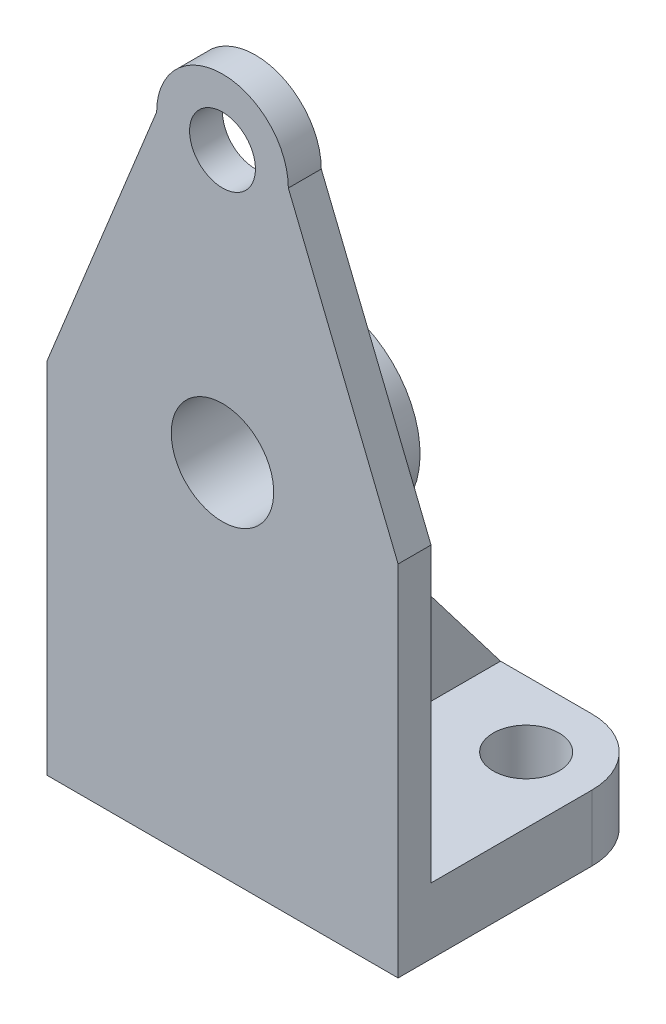
ISO-10303-21;
HEADER;
FILE_DESCRIPTION(('STEP AP214'),'2;1');
FILE_NAME('part.step','',(''),(''),'','','');
FILE_SCHEMA(('AUTOMOTIVE_DESIGN { 1 0 10303 214 1 1 1 1 }'));
ENDSEC;
DATA;
#1=APPLICATION_CONTEXT('core data for automotive mechanical design processes');
#2=APPLICATION_PROTOCOL_DEFINITION('international standard','automotive_design',2000,#1);
#3=PRODUCT_CONTEXT('',#1,'mechanical');
#4=PRODUCT('Part','Part','',(#3));
#5=PRODUCT_RELATED_PRODUCT_CATEGORY('part','',(#4));
#6=PRODUCT_DEFINITION_FORMATION('','',#4);
#7=PRODUCT_DEFINITION_CONTEXT('part definition',#1,'design');
#8=PRODUCT_DEFINITION('design','',#6,#7);
#9=PRODUCT_DEFINITION_SHAPE('','',#8);
#10=(LENGTH_UNIT() NAMED_UNIT(*) SI_UNIT(.MILLI.,.METRE.));
#11=(NAMED_UNIT(*) PLANE_ANGLE_UNIT() SI_UNIT($,.RADIAN.));
#12=(NAMED_UNIT(*) SI_UNIT($,.STERADIAN.) SOLID_ANGLE_UNIT());
#13=UNCERTAINTY_MEASURE_WITH_UNIT(LENGTH_MEASURE(1.E-05),#10,'distance_accuracy_value','');
#14=(GEOMETRIC_REPRESENTATION_CONTEXT(3) GLOBAL_UNCERTAINTY_ASSIGNED_CONTEXT((#13)) GLOBAL_UNIT_ASSIGNED_CONTEXT((#10,
#11,#12)) REPRESENTATION_CONTEXT('',''));
#15=CARTESIAN_POINT('',(0.,0.,0.));
#16=DIRECTION('',(0.,0.,1.));
#17=DIRECTION('',(1.,0.,0.));
#18=AXIS2_PLACEMENT_3D('',#15,#16,#17);
#19=CARTESIAN_POINT('',(18.,18.,-53.));
#20=DIRECTION('',(0.,-1.,0.));
#21=DIRECTION('',(0.,0.,-1.));
#22=AXIS2_PLACEMENT_3D('',#19,#20,#21);
#23=PLANE('',#22);
#24=CARTESIAN_POINT('',(18.,18.,-53.));
#25=DIRECTION('',(0.,-1.,0.));
#26=DIRECTION('',(0.,0.,-1.));
#27=AXIS2_PLACEMENT_3D('',#24,#25,#26);
#28=CIRCLE('',#27,9.);
#29=CARTESIAN_POINT('',(18.,18.,-62.));
#30=VERTEX_POINT('',#29);
#31=EDGE_CURVE('E219',#30,#30,#28,.T.);
#32=ORIENTED_EDGE('',*,*,#31,.T.);
#33=EDGE_LOOP('',(#32));
#34=FACE_BOUND('',#33,.T.);
#35=DIRECTION('',(0.,0.,1.));
#36=VECTOR('',#35,1.);
#37=CARTESIAN_POINT('',(43.,18.,-53.));
#38=LINE('',#37,#36);
#39=CARTESIAN_POINT('',(43.,18.,-71.));
#40=VERTEX_POINT('',#39);
#41=CARTESIAN_POINT('',(43.,18.,-9.));
#42=VERTEX_POINT('',#41);
#43=EDGE_CURVE('E88',#40,#42,#38,.T.);
#44=ORIENTED_EDGE('',*,*,#43,.F.);
#45=DIRECTION('',(-1.,0.,0.));
#46=VECTOR('',#45,1.);
#47=CARTESIAN_POINT('',(18.,18.,-71.));
#48=LINE('',#47,#46);
#49=CARTESIAN_POINT('',(18.,18.,-71.));
#50=VERTEX_POINT('',#49);
#51=EDGE_CURVE('E279',#40,#50,#48,.T.);
#52=ORIENTED_EDGE('',*,*,#51,.T.);
#53=CARTESIAN_POINT('',(18.,18.,-53.));
#54=DIRECTION('',(0.,1.,0.));
#55=DIRECTION('',(0.,0.,-1.));
#56=AXIS2_PLACEMENT_3D('',#53,#54,#55);
#57=CIRCLE('',#56,18.);
#58=CARTESIAN_POINT('',(0.,18.,-53.));
#59=VERTEX_POINT('',#58);
#60=EDGE_CURVE('E283',#50,#59,#57,.T.);
#61=ORIENTED_EDGE('',*,*,#60,.T.);
#62=DIRECTION('',(0.,0.,1.));
#63=VECTOR('',#62,1.);
#64=CARTESIAN_POINT('',(0.,18.,0.));
#65=LINE('',#64,#63);
#66=CARTESIAN_POINT('',(0.,18.,-9.));
#67=VERTEX_POINT('',#66);
#68=EDGE_CURVE('E281',#59,#67,#65,.T.);
#69=ORIENTED_EDGE('',*,*,#68,.T.);
#70=DIRECTION('',(-1.,0.,0.));
#71=VECTOR('',#70,1.);
#72=CARTESIAN_POINT('',(0.,18.,-9.));
#73=LINE('',#72,#71);
#74=EDGE_CURVE('E241',#42,#67,#73,.T.);
#75=ORIENTED_EDGE('',*,*,#74,.F.);
#76=EDGE_LOOP('',(#44,#52,#61,#69,#75));
#77=FACE_BOUND('',#76,.T.);
#78=ADVANCED_FACE('F72',(#34,#77),#23,.F.);
#79=CARTESIAN_POINT('',(78.,18.,-53.));
#80=DIRECTION('',(0.,-1.,0.));
#81=DIRECTION('',(0.,0.,-1.));
#82=AXIS2_PLACEMENT_3D('',#79,#80,#81);
#83=CIRCLE('',#82,9.);
#84=CARTESIAN_POINT('',(78.,18.,-62.));
#85=VERTEX_POINT('',#84);
#86=EDGE_CURVE('E214',#85,#85,#83,.T.);
#87=ORIENTED_EDGE('',*,*,#86,.T.);
#88=EDGE_LOOP('',(#87));
#89=FACE_BOUND('',#88,.T.);
#90=CARTESIAN_POINT('',(78.,18.,-71.));
#91=VERTEX_POINT('',#90);
#92=CARTESIAN_POINT('',(53.,18.,-71.));
#93=VERTEX_POINT('',#92);
#94=EDGE_CURVE('E276',#91,#93,#48,.T.);
#95=ORIENTED_EDGE('',*,*,#94,.T.);
#96=DIRECTION('',(0.,0.,1.));
#97=VECTOR('',#96,1.);
#98=CARTESIAN_POINT('',(53.,18.,-53.));
#99=LINE('',#98,#97);
#100=CARTESIAN_POINT('',(53.,18.,-9.));
#101=VERTEX_POINT('',#100);
#102=EDGE_CURVE('E198',#93,#101,#99,.T.);
#103=ORIENTED_EDGE('',*,*,#102,.T.);
#104=CARTESIAN_POINT('',(96.,18.,-9.00000000000001));
#105=VERTEX_POINT('',#104);
#106=EDGE_CURVE('E242',#105,#101,#73,.T.);
#107=ORIENTED_EDGE('',*,*,#106,.F.);
#108=DIRECTION('',(0.,0.,-1.));
#109=VECTOR('',#108,1.);
#110=CARTESIAN_POINT('',(96.,18.,-53.));
#111=LINE('',#110,#109);
#112=CARTESIAN_POINT('',(96.,18.,-53.));
#113=VERTEX_POINT('',#112);
#114=EDGE_CURVE('E272',#105,#113,#111,.T.);
#115=ORIENTED_EDGE('',*,*,#114,.T.);
#116=CARTESIAN_POINT('',(78.,18.,-53.));
#117=DIRECTION('',(0.,1.,0.));
#118=DIRECTION('',(0.,0.,-1.));
#119=AXIS2_PLACEMENT_3D('',#116,#117,#118);
#120=CIRCLE('',#119,18.);
#121=EDGE_CURVE('E274',#113,#91,#120,.T.);
#122=ORIENTED_EDGE('',*,*,#121,.T.);
#123=EDGE_LOOP('',(#95,#103,#107,#115,#122));
#124=FACE_BOUND('',#123,.T.);
#125=ADVANCED_FACE('F355',(#89,#124),#23,.F.);
#126=CARTESIAN_POINT('',(96.,18.,0.));
#127=DIRECTION('',(0.,0.,-1.));
#128=DIRECTION('',(-1.,0.,0.));
#129=AXIS2_PLACEMENT_3D('',#126,#127,#128);
#130=PLANE('',#129);
#131=DIRECTION('',(1.,0.,0.));
#132=VECTOR('',#131,1.);
#133=CARTESIAN_POINT('',(96.,0.,0.));
#134=LINE('',#133,#132);
#135=CARTESIAN_POINT('',(0.,0.,0.));
#136=VERTEX_POINT('',#135);
#137=CARTESIAN_POINT('',(96.,0.,0.));
#138=VERTEX_POINT('',#137);
#139=EDGE_CURVE('E261',#136,#138,#134,.T.);
#140=ORIENTED_EDGE('',*,*,#139,.T.);
#141=DIRECTION('',(0.,-1.,0.));
#142=VECTOR('',#141,1.);
#143=CARTESIAN_POINT('',(96.,18.,0.));
#144=LINE('',#143,#142);
#145=CARTESIAN_POINT('',(96.,98.,0.));
#146=VERTEX_POINT('',#145);
#147=EDGE_CURVE('E77',#146,#138,#144,.T.);
#148=ORIENTED_EDGE('',*,*,#147,.F.);
#149=DIRECTION('',(0.375705108739218,-0.926739268223405,0.));
#150=VECTOR('',#149,1.);
#151=CARTESIAN_POINT('',(116.570890840652,47.2584692597239,0.));
#152=LINE('',#151,#150);
#153=CARTESIAN_POINT('',(66.,172.,0.));
#154=VERTEX_POINT('',#153);
#155=EDGE_CURVE('E243',#154,#146,#152,.T.);
#156=ORIENTED_EDGE('',*,*,#155,.F.);
#157=CARTESIAN_POINT('',(48.,172.,0.));
#158=DIRECTION('',(0.,0.,1.));
#159=DIRECTION('',(1.,0.,0.));
#160=AXIS2_PLACEMENT_3D('',#157,#158,#159);
#161=CIRCLE('',#160,18.);
#162=CARTESIAN_POINT('',(30.,172.,0.));
#163=VERTEX_POINT('',#162);
#164=EDGE_CURVE('E231',#154,#163,#161,.T.);
#165=ORIENTED_EDGE('',*,*,#164,.T.);
#166=DIRECTION('',(-0.375705108739218,-0.926739268223405,0.));
#167=VECTOR('',#166,1.);
#168=CARTESIAN_POINT('',(-34.1217063989962,13.8331242158093,0.));
#169=LINE('',#168,#167);
#170=CARTESIAN_POINT('',(0.,98.,0.));
#171=VERTEX_POINT('',#170);
#172=EDGE_CURVE('E251',#163,#171,#169,.T.);
#173=ORIENTED_EDGE('',*,*,#172,.T.);
#174=DIRECTION('',(0.,-1.,0.));
#175=VECTOR('',#174,1.);
#176=CARTESIAN_POINT('',(0.,18.,0.));
#177=LINE('',#176,#175);
#178=EDGE_CURVE('E287',#171,#136,#177,.T.);
#179=ORIENTED_EDGE('',*,*,#178,.T.);
#180=EDGE_LOOP('',(#140,#148,#156,#165,#173,#179));
#181=FACE_BOUND('',#180,.T.);
#182=CARTESIAN_POINT('',(48.,98.,0.));
#183=DIRECTION('',(0.,0.,-1.));
#184=DIRECTION('',(-1.,0.,0.));
#185=AXIS2_PLACEMENT_3D('',#182,#183,#184);
#186=CIRCLE('',#185,14.);
#187=CARTESIAN_POINT('',(34.,98.,0.));
#188=VERTEX_POINT('',#187);
#189=EDGE_CURVE('E221',#188,#188,#186,.T.);
#190=ORIENTED_EDGE('',*,*,#189,.T.);
#191=EDGE_LOOP('',(#190));
#192=FACE_BOUND('',#191,.T.);
#193=CARTESIAN_POINT('',(48.,172.,0.));
#194=DIRECTION('',(0.,0.,-1.));
#195=DIRECTION('',(-1.,0.,0.));
#196=AXIS2_PLACEMENT_3D('',#193,#194,#195);
#197=CIRCLE('',#196,9.00000000000001);
#198=CARTESIAN_POINT('',(39.,172.,0.));
#199=VERTEX_POINT('',#198);
#200=EDGE_CURVE('E232',#199,#199,#197,.T.);
#201=ORIENTED_EDGE('',*,*,#200,.T.);
#202=EDGE_LOOP('',(#201));
#203=FACE_BOUND('',#202,.T.);
#204=ADVANCED_FACE('F71',(#181,#192,#203),#130,.F.);
#205=CARTESIAN_POINT('',(96.,18.,-53.));
#206=DIRECTION('',(-1.,0.,0.));
#207=DIRECTION('',(0.,0.,1.));
#208=AXIS2_PLACEMENT_3D('',#205,#206,#207);
#209=PLANE('',#208);
#210=DIRECTION('',(0.,0.,-1.));
#211=VECTOR('',#210,1.);
#212=CARTESIAN_POINT('',(96.,0.,-53.));
#213=LINE('',#212,#211);
#214=CARTESIAN_POINT('',(96.,0.,-53.));
#215=VERTEX_POINT('',#214);
#216=EDGE_CURVE('E289',#138,#215,#213,.T.);
#217=ORIENTED_EDGE('',*,*,#216,.T.);
#218=DIRECTION('',(0.,-1.,0.));
#219=VECTOR('',#218,1.);
#220=CARTESIAN_POINT('',(96.,18.,-53.));
#221=LINE('',#220,#219);
#222=EDGE_CURVE('E306',#113,#215,#221,.T.);
#223=ORIENTED_EDGE('',*,*,#222,.F.);
#224=ORIENTED_EDGE('',*,*,#114,.F.);
#225=DIRECTION('',(0.,-1.,0.));
#226=VECTOR('',#225,1.);
#227=CARTESIAN_POINT('',(96.,0.,-9.));
#228=LINE('',#227,#226);
#229=CARTESIAN_POINT('',(96.,98.,-9.));
#230=VERTEX_POINT('',#229);
#231=EDGE_CURVE('E250',#230,#105,#228,.T.);
#232=ORIENTED_EDGE('',*,*,#231,.F.);
#233=DIRECTION('',(0.,0.,1.));
#234=VECTOR('',#233,1.);
#235=CARTESIAN_POINT('',(96.,98.,-9.));
#236=LINE('',#235,#234);
#237=EDGE_CURVE('E265',#230,#146,#236,.T.);
#238=ORIENTED_EDGE('',*,*,#237,.T.);
#239=ORIENTED_EDGE('',*,*,#147,.T.);
#240=EDGE_LOOP('',(#217,#223,#224,#232,#238,#239));
#241=FACE_BOUND('',#240,.T.);
#242=ADVANCED_FACE('F315',(#241),#209,.F.);
#243=CARTESIAN_POINT('',(78.,18.,-53.));
#244=DIRECTION('',(0.,-1.,0.));
#245=DIRECTION('',(0.,0.,-1.));
#246=AXIS2_PLACEMENT_3D('',#243,#244,#245);
#247=CYLINDRICAL_SURFACE('',#246,18.);
#248=CARTESIAN_POINT('',(78.,0.,-53.));
#249=DIRECTION('',(0.,1.,0.));
#250=DIRECTION('',(0.,0.,-1.));
#251=AXIS2_PLACEMENT_3D('',#248,#249,#250);
#252=CIRCLE('',#251,18.);
#253=CARTESIAN_POINT('',(78.,0.,-71.));
#254=VERTEX_POINT('',#253);
#255=EDGE_CURVE('E288',#215,#254,#252,.T.);
#256=ORIENTED_EDGE('',*,*,#255,.T.);
#257=DIRECTION('',(0.,-1.,0.));
#258=VECTOR('',#257,1.);
#259=CARTESIAN_POINT('',(78.,18.,-71.));
#260=LINE('',#259,#258);
#261=EDGE_CURVE('E303',#91,#254,#260,.T.);
#262=ORIENTED_EDGE('',*,*,#261,.F.);
#263=ORIENTED_EDGE('',*,*,#121,.F.);
#264=ORIENTED_EDGE('',*,*,#222,.T.);
#265=EDGE_LOOP('',(#256,#262,#263,#264));
#266=FACE_BOUND('',#265,.T.);
#267=ADVANCED_FACE('F347',(#266),#247,.T.);
#268=CARTESIAN_POINT('',(18.,18.,-71.));
#269=DIRECTION('',(0.,0.,1.));
#270=DIRECTION('',(1.,0.,0.));
#271=AXIS2_PLACEMENT_3D('',#268,#269,#270);
#272=PLANE('',#271);
#273=DIRECTION('',(-1.,0.,0.));
#274=VECTOR('',#273,1.);
#275=CARTESIAN_POINT('',(18.,0.,-71.));
#276=LINE('',#275,#274);
#277=CARTESIAN_POINT('',(18.,0.,-71.));
#278=VERTEX_POINT('',#277);
#279=EDGE_CURVE('E295',#254,#278,#276,.T.);
#280=ORIENTED_EDGE('',*,*,#279,.T.);
#281=DIRECTION('',(0.,-1.,0.));
#282=VECTOR('',#281,1.);
#283=CARTESIAN_POINT('',(18.,18.,-71.));
#284=LINE('',#283,#282);
#285=EDGE_CURVE('E305',#50,#278,#284,.T.);
#286=ORIENTED_EDGE('',*,*,#285,.F.);
#287=ORIENTED_EDGE('',*,*,#51,.F.);
#288=DIRECTION('',(1.,0.,0.));
#289=VECTOR('',#288,1.);
#290=CARTESIAN_POINT('',(18.,18.,-71.));
#291=LINE('',#290,#289);
#292=EDGE_CURVE('E91',#93,#40,#291,.F.);
#293=ORIENTED_EDGE('',*,*,#292,.F.);
#294=ORIENTED_EDGE('',*,*,#94,.F.);
#295=ORIENTED_EDGE('',*,*,#261,.T.);
#296=EDGE_LOOP('',(#280,#286,#287,#293,#294,#295));
#297=FACE_BOUND('',#296,.T.);
#298=ADVANCED_FACE('F346',(#297),#272,.F.);
#299=CARTESIAN_POINT('',(18.,18.,-53.));
#300=DIRECTION('',(0.,-1.,0.));
#301=DIRECTION('',(0.,0.,-1.));
#302=AXIS2_PLACEMENT_3D('',#299,#300,#301);
#303=CYLINDRICAL_SURFACE('',#302,18.);
#304=CARTESIAN_POINT('',(18.,0.,-53.));
#305=DIRECTION('',(0.,1.,0.));
#306=DIRECTION('',(0.,0.,-1.));
#307=AXIS2_PLACEMENT_3D('',#304,#305,#306);
#308=CIRCLE('',#307,18.);
#309=CARTESIAN_POINT('',(0.,0.,-53.));
#310=VERTEX_POINT('',#309);
#311=EDGE_CURVE('E294',#278,#310,#308,.T.);
#312=ORIENTED_EDGE('',*,*,#311,.T.);
#313=DIRECTION('',(0.,-1.,0.));
#314=VECTOR('',#313,1.);
#315=CARTESIAN_POINT('',(0.,18.,-53.));
#316=LINE('',#315,#314);
#317=EDGE_CURVE('E297',#59,#310,#316,.T.);
#318=ORIENTED_EDGE('',*,*,#317,.F.);
#319=ORIENTED_EDGE('',*,*,#60,.F.);
#320=ORIENTED_EDGE('',*,*,#285,.T.);
#321=EDGE_LOOP('',(#312,#318,#319,#320));
#322=FACE_BOUND('',#321,.T.);
#323=ADVANCED_FACE('F386',(#322),#303,.T.);
#324=CARTESIAN_POINT('',(0.,18.,0.));
#325=DIRECTION('',(1.,0.,0.));
#326=DIRECTION('',(0.,0.,-1.));
#327=AXIS2_PLACEMENT_3D('',#324,#325,#326);
#328=PLANE('',#327);
#329=DIRECTION('',(0.,0.,1.));
#330=VECTOR('',#329,1.);
#331=CARTESIAN_POINT('',(0.,0.,0.));
#332=LINE('',#331,#330);
#333=EDGE_CURVE('E277',#310,#136,#332,.T.);
#334=ORIENTED_EDGE('',*,*,#333,.T.);
#335=ORIENTED_EDGE('',*,*,#178,.F.);
#336=DIRECTION('',(0.,0.,1.));
#337=VECTOR('',#336,1.);
#338=CARTESIAN_POINT('',(0.,98.,-9.));
#339=LINE('',#338,#337);
#340=CARTESIAN_POINT('',(0.,98.,-9.));
#341=VERTEX_POINT('',#340);
#342=EDGE_CURVE('E264',#341,#171,#339,.T.);
#343=ORIENTED_EDGE('',*,*,#342,.F.);
#344=DIRECTION('',(0.,1.,0.));
#345=VECTOR('',#344,1.);
#346=CARTESIAN_POINT('',(0.,0.,-9.));
#347=LINE('',#346,#345);
#348=EDGE_CURVE('E238',#67,#341,#347,.T.);
#349=ORIENTED_EDGE('',*,*,#348,.F.);
#350=ORIENTED_EDGE('',*,*,#68,.F.);
#351=ORIENTED_EDGE('',*,*,#317,.T.);
#352=EDGE_LOOP('',(#334,#335,#343,#349,#350,#351));
#353=FACE_BOUND('',#352,.T.);
#354=ADVANCED_FACE('F333',(#353),#328,.F.);
#355=CARTESIAN_POINT('',(18.,0.,-53.));
#356=DIRECTION('',(0.,-1.,0.));
#357=DIRECTION('',(0.,0.,-1.));
#358=AXIS2_PLACEMENT_3D('',#355,#356,#357);
#359=PLANE('',#358);
#360=ORIENTED_EDGE('',*,*,#216,.F.);
#361=ORIENTED_EDGE('',*,*,#139,.F.);
#362=ORIENTED_EDGE('',*,*,#333,.F.);
#363=ORIENTED_EDGE('',*,*,#311,.F.);
#364=ORIENTED_EDGE('',*,*,#279,.F.);
#365=ORIENTED_EDGE('',*,*,#255,.F.);
#366=EDGE_LOOP('',(#360,#361,#362,#363,#364,#365));
#367=FACE_BOUND('',#366,.T.);
#368=CARTESIAN_POINT('',(78.,0.,-53.));
#369=DIRECTION('',(0.,-1.,0.));
#370=DIRECTION('',(0.,0.,-1.));
#371=AXIS2_PLACEMENT_3D('',#368,#369,#370);
#372=CIRCLE('',#371,9.);
#373=CARTESIAN_POINT('',(78.,0.,-62.));
#374=VERTEX_POINT('',#373);
#375=EDGE_CURVE('E211',#374,#374,#372,.T.);
#376=ORIENTED_EDGE('',*,*,#375,.F.);
#377=EDGE_LOOP('',(#376));
#378=FACE_BOUND('',#377,.T.);
#379=CARTESIAN_POINT('',(18.,0.,-53.));
#380=DIRECTION('',(0.,-1.,0.));
#381=DIRECTION('',(0.,0.,-1.));
#382=AXIS2_PLACEMENT_3D('',#379,#380,#381);
#383=CIRCLE('',#382,9.);
#384=CARTESIAN_POINT('',(18.,0.,-62.));
#385=VERTEX_POINT('',#384);
#386=EDGE_CURVE('E215',#385,#385,#383,.T.);
#387=ORIENTED_EDGE('',*,*,#386,.F.);
#388=EDGE_LOOP('',(#387));
#389=FACE_BOUND('',#388,.T.);
#390=ADVANCED_FACE('F337',(#367,#378,#389),#359,.T.);
#391=CARTESIAN_POINT('',(116.570890840652,47.2584692597239,-9.));
#392=DIRECTION('',(-0.926739268223405,-0.375705108739218,0.));
#393=DIRECTION('',(0.375705108739218,-0.926739268223405,0.));
#394=AXIS2_PLACEMENT_3D('',#391,#392,#393);
#395=PLANE('',#394);
#396=ORIENTED_EDGE('',*,*,#155,.T.);
#397=ORIENTED_EDGE('',*,*,#237,.F.);
#398=DIRECTION('',(0.375705108739218,-0.926739268223405,0.));
#399=VECTOR('',#398,1.);
#400=CARTESIAN_POINT('',(116.570890840652,47.2584692597239,-9.));
#401=LINE('',#400,#399);
#402=CARTESIAN_POINT('',(66.,172.,-9.));
#403=VERTEX_POINT('',#402);
#404=EDGE_CURVE('E248',#403,#230,#401,.T.);
#405=ORIENTED_EDGE('',*,*,#404,.F.);
#406=DIRECTION('',(0.,0.,1.));
#407=VECTOR('',#406,1.);
#408=CARTESIAN_POINT('',(66.,172.,-9.));
#409=LINE('',#408,#407);
#410=EDGE_CURVE('E259',#403,#154,#409,.T.);
#411=ORIENTED_EDGE('',*,*,#410,.T.);
#412=EDGE_LOOP('',(#396,#397,#405,#411));
#413=FACE_BOUND('',#412,.T.);
#414=ADVANCED_FACE('F325',(#413),#395,.F.);
#415=CARTESIAN_POINT('',(-34.1217063989962,13.8331242158093,-9.));
#416=DIRECTION('',(-0.926739268223405,0.375705108739218,0.));
#417=DIRECTION('',(-0.375705108739218,-0.926739268223405,0.));
#418=AXIS2_PLACEMENT_3D('',#415,#416,#417);
#419=PLANE('',#418);
#420=ORIENTED_EDGE('',*,*,#172,.F.);
#421=DIRECTION('',(0.,0.,1.));
#422=VECTOR('',#421,1.);
#423=CARTESIAN_POINT('',(30.,172.,-9.));
#424=LINE('',#423,#422);
#425=CARTESIAN_POINT('',(30.,172.,-9.));
#426=VERTEX_POINT('',#425);
#427=EDGE_CURVE('E252',#426,#163,#424,.T.);
#428=ORIENTED_EDGE('',*,*,#427,.F.);
#429=DIRECTION('',(-0.375705108739218,-0.926739268223405,0.));
#430=VECTOR('',#429,1.);
#431=CARTESIAN_POINT('',(-34.1217063989962,13.8331242158093,-9.));
#432=LINE('',#431,#430);
#433=EDGE_CURVE('E240',#426,#341,#432,.T.);
#434=ORIENTED_EDGE('',*,*,#433,.T.);
#435=ORIENTED_EDGE('',*,*,#342,.T.);
#436=EDGE_LOOP('',(#420,#428,#434,#435));
#437=FACE_BOUND('',#436,.T.);
#438=ADVANCED_FACE('F329',(#437),#419,.T.);
#439=CARTESIAN_POINT('',(0.,0.,-9.));
#440=DIRECTION('',(0.,0.,1.));
#441=DIRECTION('',(1.,0.,0.));
#442=AXIS2_PLACEMENT_3D('',#439,#440,#441);
#443=PLANE('',#442);
#444=CARTESIAN_POINT('',(48.,172.,-9.));
#445=DIRECTION('',(0.,0.,-1.));
#446=DIRECTION('',(-1.,0.,0.));
#447=AXIS2_PLACEMENT_3D('',#444,#445,#446);
#448=CIRCLE('',#447,9.00000000000001);
#449=CARTESIAN_POINT('',(39.,172.,-9.));
#450=VERTEX_POINT('',#449);
#451=EDGE_CURVE('E229',#450,#450,#448,.T.);
#452=ORIENTED_EDGE('',*,*,#451,.F.);
#453=EDGE_LOOP('',(#452));
#454=FACE_BOUND('',#453,.T.);
#455=ORIENTED_EDGE('',*,*,#106,.T.);
#456=DIRECTION('',(0.,1.,0.));
#457=VECTOR('',#456,1.);
#458=CARTESIAN_POINT('',(53.,0.,-9.));
#459=LINE('',#458,#457);
#460=CARTESIAN_POINT('',(53.,73.5051025721682,-9.));
#461=VERTEX_POINT('',#460);
#462=EDGE_CURVE('E210',#101,#461,#459,.T.);
#463=ORIENTED_EDGE('',*,*,#462,.T.);
#464=CARTESIAN_POINT('',(48.,98.,-9.));
#465=DIRECTION('',(0.,0.,1.));
#466=DIRECTION('',(1.,0.,0.));
#467=AXIS2_PLACEMENT_3D('',#464,#465,#466);
#468=CIRCLE('',#467,25.);
#469=CARTESIAN_POINT('',(43.,73.5051025721682,-9.));
#470=VERTEX_POINT('',#469);
#471=EDGE_CURVE('E12',#470,#461,#468,.F.);
#472=ORIENTED_EDGE('',*,*,#471,.F.);
#473=DIRECTION('',(0.,1.,0.));
#474=VECTOR('',#473,1.);
#475=CARTESIAN_POINT('',(43.,0.,-9.));
#476=LINE('',#475,#474);
#477=EDGE_CURVE('E193',#42,#470,#476,.T.);
#478=ORIENTED_EDGE('',*,*,#477,.F.);
#479=ORIENTED_EDGE('',*,*,#74,.T.);
#480=ORIENTED_EDGE('',*,*,#348,.T.);
#481=ORIENTED_EDGE('',*,*,#433,.F.);
#482=CARTESIAN_POINT('',(48.,172.,-9.));
#483=DIRECTION('',(0.,0.,1.));
#484=DIRECTION('',(1.,0.,0.));
#485=AXIS2_PLACEMENT_3D('',#482,#483,#484);
#486=CIRCLE('',#485,18.);
#487=EDGE_CURVE('E258',#403,#426,#486,.T.);
#488=ORIENTED_EDGE('',*,*,#487,.F.);
#489=ORIENTED_EDGE('',*,*,#404,.T.);
#490=ORIENTED_EDGE('',*,*,#231,.T.);
#491=EDGE_LOOP('',(#455,#463,#472,#478,#479,#480,#481,#488,#489,#490));
#492=FACE_BOUND('',#491,.T.);
#493=ADVANCED_FACE('F425',(#454,#492),#443,.F.);
#494=CARTESIAN_POINT('',(48.,172.,-9.));
#495=DIRECTION('',(0.,0.,1.));
#496=DIRECTION('',(1.,0.,0.));
#497=AXIS2_PLACEMENT_3D('',#494,#495,#496);
#498=CYLINDRICAL_SURFACE('',#497,18.);
#499=ORIENTED_EDGE('',*,*,#410,.F.);
#500=ORIENTED_EDGE('',*,*,#487,.T.);
#501=ORIENTED_EDGE('',*,*,#427,.T.);
#502=ORIENTED_EDGE('',*,*,#164,.F.);
#503=EDGE_LOOP('',(#499,#500,#501,#502));
#504=FACE_BOUND('',#503,.T.);
#505=ADVANCED_FACE('F330',(#504),#498,.T.);
#506=CARTESIAN_POINT('',(48.,172.,0.));
#507=DIRECTION('',(0.,0.,-1.));
#508=DIRECTION('',(-1.,0.,0.));
#509=AXIS2_PLACEMENT_3D('',#506,#507,#508);
#510=CYLINDRICAL_SURFACE('',#509,9.00000000000001);
#511=ORIENTED_EDGE('',*,*,#200,.F.);
#512=EDGE_LOOP('',(#511));
#513=FACE_BOUND('',#512,.T.);
#514=ORIENTED_EDGE('',*,*,#451,.T.);
#515=EDGE_LOOP('',(#514));
#516=FACE_BOUND('',#515,.T.);
#517=ADVANCED_FACE('F371',(#513,#516),#510,.F.);
#518=CARTESIAN_POINT('',(48.,98.,-29.));
#519=DIRECTION('',(0.,0.,1.));
#520=DIRECTION('',(1.,0.,0.));
#521=AXIS2_PLACEMENT_3D('',#518,#519,#520);
#522=CYLINDRICAL_SURFACE('',#521,25.);
#523=ORIENTED_EDGE('',*,*,#471,.T.);
#524=DIRECTION('',(0.,0.,1.));
#525=VECTOR('',#524,1.);
#526=CARTESIAN_POINT('',(53.,73.5051025721682,-29.));
#527=LINE('',#526,#525);
#528=CARTESIAN_POINT('',(53.,73.5051025721682,-28.6142853085261));
#529=VERTEX_POINT('',#528);
#530=EDGE_CURVE('E186',#461,#529,#527,.F.);
#531=ORIENTED_EDGE('',*,*,#530,.T.);
#532=CARTESIAN_POINT('',(48.,98.,-9.9090909090909));
#533=DIRECTION('',(0.,-0.60691360336223,0.79476781392673));
#534=DIRECTION('',(0.,0.79476781392673,0.60691360336223));
#535=AXIS2_PLACEMENT_3D('',#532,#533,#534);
#536=ELLIPSE('',#535,31.4557277759926,25.);
#537=CARTESIAN_POINT('',(48.,73.,-29.));
#538=VERTEX_POINT('',#537);
#539=EDGE_CURVE('E190',#529,#538,#536,.F.);
#540=ORIENTED_EDGE('',*,*,#539,.T.);
#541=CARTESIAN_POINT('',(48.,98.,-29.));
#542=DIRECTION('',(0.,0.,-1.));
#543=DIRECTION('',(-1.,0.,0.));
#544=AXIS2_PLACEMENT_3D('',#541,#542,#543);
#545=CIRCLE('',#544,25.);
#546=EDGE_CURVE('E181',#538,#538,#545,.T.);
#547=ORIENTED_EDGE('',*,*,#546,.F.);
#548=CARTESIAN_POINT('',(43.,73.5051025721682,-28.6142853085261));
#549=VERTEX_POINT('',#548);
#550=EDGE_CURVE('E180',#538,#549,#536,.F.);
#551=ORIENTED_EDGE('',*,*,#550,.T.);
#552=DIRECTION('',(0.,0.,1.));
#553=VECTOR('',#552,1.);
#554=CARTESIAN_POINT('',(43.,73.5051025721682,-29.));
#555=LINE('',#554,#553);
#556=EDGE_CURVE('E178',#470,#549,#555,.F.);
#557=ORIENTED_EDGE('',*,*,#556,.F.);
#558=EDGE_LOOP('',(#523,#531,#540,#547,#551,#557));
#559=FACE_BOUND('',#558,.T.);
#560=ADVANCED_FACE('F176',(#559),#522,.T.);
#561=CARTESIAN_POINT('',(48.,98.,-29.));
#562=DIRECTION('',(0.,0.,-1.));
#563=DIRECTION('',(-1.,0.,0.));
#564=AXIS2_PLACEMENT_3D('',#561,#562,#563);
#565=PLANE('',#564);
#566=CARTESIAN_POINT('',(48.,98.,-29.));
#567=DIRECTION('',(0.,0.,-1.));
#568=DIRECTION('',(-1.,0.,0.));
#569=AXIS2_PLACEMENT_3D('',#566,#567,#568);
#570=CIRCLE('',#569,14.);
#571=CARTESIAN_POINT('',(34.,98.,-29.));
#572=VERTEX_POINT('',#571);
#573=EDGE_CURVE('E224',#572,#572,#570,.T.);
#574=ORIENTED_EDGE('',*,*,#573,.F.);
#575=EDGE_LOOP('',(#574));
#576=FACE_BOUND('',#575,.T.);
#577=ORIENTED_EDGE('',*,*,#546,.T.);
#578=EDGE_LOOP('',(#577));
#579=FACE_BOUND('',#578,.T.);
#580=ADVANCED_FACE('F356',(#576,#579),#565,.T.);
#581=CARTESIAN_POINT('',(48.,98.,0.));
#582=DIRECTION('',(0.,0.,-1.));
#583=DIRECTION('',(-1.,0.,0.));
#584=AXIS2_PLACEMENT_3D('',#581,#582,#583);
#585=CYLINDRICAL_SURFACE('',#584,14.);
#586=ORIENTED_EDGE('',*,*,#189,.F.);
#587=EDGE_LOOP('',(#586));
#588=FACE_BOUND('',#587,.T.);
#589=ORIENTED_EDGE('',*,*,#573,.T.);
#590=EDGE_LOOP('',(#589));
#591=FACE_BOUND('',#590,.T.);
#592=ADVANCED_FACE('F363',(#588,#591),#585,.F.);
#593=CARTESIAN_POINT('',(78.,190.,-53.));
#594=DIRECTION('',(0.,-1.,0.));
#595=DIRECTION('',(0.,0.,-1.));
#596=AXIS2_PLACEMENT_3D('',#593,#594,#595);
#597=CYLINDRICAL_SURFACE('',#596,9.);
#598=ORIENTED_EDGE('',*,*,#375,.T.);
#599=EDGE_LOOP('',(#598));
#600=FACE_BOUND('',#599,.T.);
#601=ORIENTED_EDGE('',*,*,#86,.F.);
#602=EDGE_LOOP('',(#601));
#603=FACE_BOUND('',#602,.T.);
#604=ADVANCED_FACE('F366',(#600,#603),#597,.F.);
#605=CARTESIAN_POINT('',(18.,190.,-53.));
#606=DIRECTION('',(0.,-1.,0.));
#607=DIRECTION('',(0.,0.,-1.));
#608=AXIS2_PLACEMENT_3D('',#605,#606,#607);
#609=CYLINDRICAL_SURFACE('',#608,9.);
#610=ORIENTED_EDGE('',*,*,#386,.T.);
#611=EDGE_LOOP('',(#610));
#612=FACE_BOUND('',#611,.T.);
#613=ORIENTED_EDGE('',*,*,#31,.F.);
#614=EDGE_LOOP('',(#613));
#615=FACE_BOUND('',#614,.T.);
#616=ADVANCED_FACE('F459',(#612,#615),#609,.F.);
#617=CARTESIAN_POINT('',(48.,73.,-29.));
#618=DIRECTION('',(0.,-0.60691360336223,0.79476781392673));
#619=DIRECTION('',(0.,-0.79476781392673,-0.60691360336223));
#620=AXIS2_PLACEMENT_3D('',#617,#618,#619);
#621=PLANE('',#620);
#622=DIRECTION('',(0.,-0.79476781392673,-0.60691360336223));
#623=VECTOR('',#622,1.);
#624=CARTESIAN_POINT('',(53.,73.,-29.));
#625=LINE('',#624,#623);
#626=EDGE_CURVE('E199',#529,#93,#625,.T.);
#627=ORIENTED_EDGE('',*,*,#626,.T.);
#628=ORIENTED_EDGE('',*,*,#292,.T.);
#629=DIRECTION('',(0.,-0.79476781392673,-0.60691360336223));
#630=VECTOR('',#629,1.);
#631=CARTESIAN_POINT('',(43.,73.,-29.));
#632=LINE('',#631,#630);
#633=EDGE_CURVE('E191',#549,#40,#632,.T.);
#634=ORIENTED_EDGE('',*,*,#633,.F.);
#635=ORIENTED_EDGE('',*,*,#550,.F.);
#636=ORIENTED_EDGE('',*,*,#539,.F.);
#637=EDGE_LOOP('',(#627,#628,#634,#635,#636));
#638=FACE_BOUND('',#637,.T.);
#639=ADVANCED_FACE('F200',(#638),#621,.F.);
#640=CARTESIAN_POINT('',(53.,95.,-35.5));
#641=DIRECTION('',(1.,0.,0.));
#642=DIRECTION('',(0.,0.,-1.));
#643=AXIS2_PLACEMENT_3D('',#640,#641,#642);
#644=PLANE('',#643);
#645=ORIENTED_EDGE('',*,*,#530,.F.);
#646=ORIENTED_EDGE('',*,*,#462,.F.);
#647=ORIENTED_EDGE('',*,*,#102,.F.);
#648=ORIENTED_EDGE('',*,*,#626,.F.);
#649=EDGE_LOOP('',(#645,#646,#647,#648));
#650=FACE_BOUND('',#649,.T.);
#651=ADVANCED_FACE('F360',(#650),#644,.T.);
#652=CARTESIAN_POINT('',(43.,95.,-35.5));
#653=DIRECTION('',(1.,0.,0.));
#654=DIRECTION('',(0.,0.,-1.));
#655=AXIS2_PLACEMENT_3D('',#652,#653,#654);
#656=PLANE('',#655);
#657=ORIENTED_EDGE('',*,*,#477,.T.);
#658=ORIENTED_EDGE('',*,*,#556,.T.);
#659=ORIENTED_EDGE('',*,*,#633,.T.);
#660=ORIENTED_EDGE('',*,*,#43,.T.);
#661=EDGE_LOOP('',(#657,#658,#659,#660));
#662=FACE_BOUND('',#661,.T.);
#663=ADVANCED_FACE('F194',(#662),#656,.F.);
#664=CLOSED_SHELL('',(#78,#125,#204,#242,#267,#298,#323,#354,#390,#414,#438,#493,#505,#517,#560,
#580,#592,#604,#616,#639,#651,#663));
#665=MANIFOLD_SOLID_BREP('B2',#664);
#666=ADVANCED_BREP_SHAPE_REPRESENTATION('',(#18,#665),#14);
#667=SHAPE_DEFINITION_REPRESENTATION(#9,#666);
ENDSEC;
END-ISO-10303-21;
